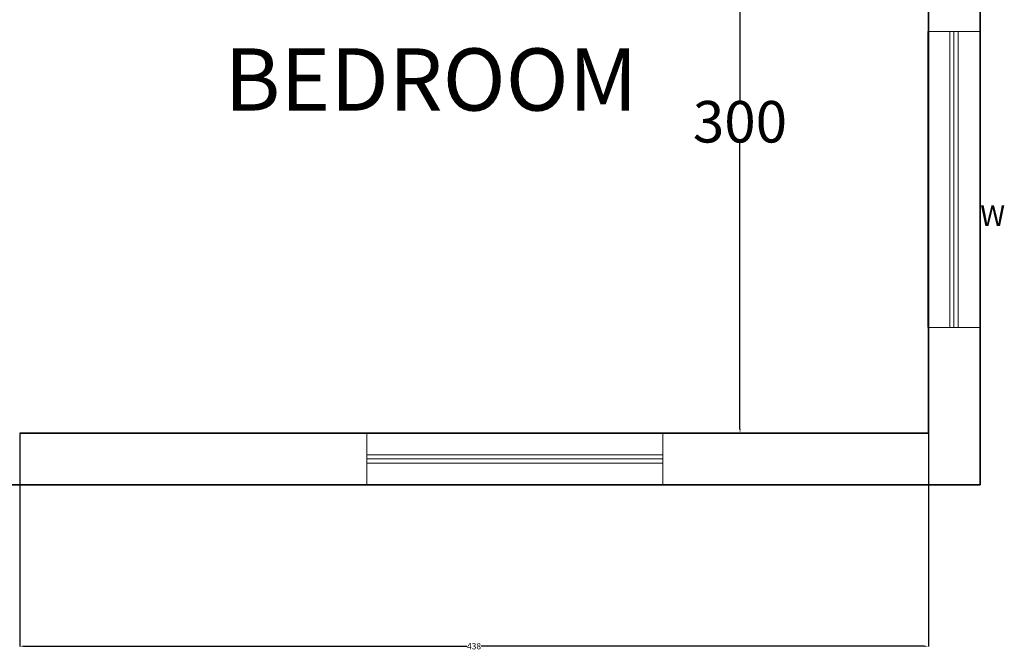
# Model space of a CAD drawing. Units: centimetres. Extents: x -121 to 3851, y -16 to 1180.
# Tile 14 of 16: x 3304 to 3779, y 16 to 320. Entities that reach past the tile are written whole.
import ezdxf

# ---------------------------------------------------------------- set-up
doc = ezdxf.new("R2010")
doc.units = ezdxf.units.CM
doc.header["$MEASUREMENT"] = 0
for name, color, linetype, lineweight in [('A-ANNO-DIMS', 2, 'Continuous', 18), ('A-ANNO-IDEN', 3, 'Continuous', 13), ('A-AREA-IDEN', 3, 'Continuous', 18), ('A-GLAZ', 4, 'Continuous', 18), ('A-WALL', 7, 'Continuous', 35)]:
    doc.layers.add(name, color=color, linetype=linetype, lineweight=lineweight)
doc.styles.get("Standard").update_dxf_attribs({"font": 'arial.ttf'})
doc.dimstyles.get("Standard").update_dxf_attribs({"dimtxt": 3, "dimasz": 2, "dimexe": 0.18, "dimexo": 0.0625, "dimgap": 0.09, "dimtad": 0, "dimtih": 1, "dimtoh": 1, "dimdec": 0, "dimzin": 0, "dimdsep": 46, "dimtxsty": 'Standard', "dimcen": 0.09, "dimadec": 0, "dimazin": 0, "dimtfac": 1, "dimtdec": 0, "dimtofl": 0, "dimtmove": 0, "dimatfit": 3, "dimfxl": 1, "dimtolj": 1, "dimtzin": 0, "dimarcsym": 0})

# ---------------------------------------------------------------- blocks, each defined once
blk = doc.blocks.new('*D17')
at = {"layer": 'A-ANNO-DIMS', "color": 0, "lineweight": -2, "transparency": 16777216}
for p, q in [((3651.46, 418.72), (3651.46, 281.03)), ((3651.53, 420.72), (3651.64, 420.72)), ((3651.46, 122.72), (3651.46, 260.41)), ((3651.53, 120.72), (3651.64, 120.72))]:
    blk.add_line(p, q, dxfattribs=at)
at = {"layer": 'A-ANNO-DIMS', "color": 0, "transparency": 16777216}
for points in [[(3651.13, 418.72), (3651.8, 418.72), (3651.46, 420.72)], [(3651.13, 122.72), (3651.8, 122.72), (3651.46, 120.72)]]:
    blk.add_solid(points, dxfattribs=at)
at = {"layer": 'Defpoints', "color": 0, "transparency": 16777216}
for p in [(3651.46, 420.72), (3651.46, 120.72), (3651.46, 120.72)]:
    blk.add_point(p, dxfattribs=at)
at = {"layer": 'A-ANNO-DIMS', "color": 0, "transparency": 16777216, "insert": (3651.46, 270.72), "char_height": 3, "attachment_point": 5}
blk.add_mtext('\\A1;{\\H6.66667x;300}', dxfattribs=at)
blk = doc.blocks.new('WIN-143CM')
for p, q in [((0, 14.5), (142.63, 14.5)), ((0, 12.5), (142.63, 12.5)), ((0, 10.5), (142.63, 10.5))]:
    blk.add_line(p, q)
blk.add_lwpolyline([(0, 25), (142.63, 25), (142.63, 0), (0, 0)], close=True)
blk = doc.blocks.new('*D64')
at = {"layer": 'A-ANNO-DIMS', "color": 0, "lineweight": -2, "transparency": 16777216}
for p, q in [((3304.26, 120.66), (3304.26, 17.79)), ((3742.26, 120.66), (3742.26, 17.79)), ((3306.26, 17.97), (3519.8, 17.97)), ((3740.26, 17.97), (3526.73, 17.97))]:
    blk.add_line(p, q, dxfattribs=at)
at = {"layer": 'A-ANNO-DIMS', "color": 0, "transparency": 16777216}
for points in [[(3306.26, 18.31), (3306.26, 17.64), (3304.26, 17.97)], [(3740.26, 18.31), (3740.26, 17.64), (3742.26, 17.97)]]:
    blk.add_solid(points, dxfattribs=at)
at = {"layer": 'Defpoints', "color": 0, "transparency": 16777216}
for p in [(3304.26, 120.72), (3742.26, 120.72), (3742.26, 17.97)]:
    blk.add_point(p, dxfattribs=at)
at = {"layer": 'A-ANNO-DIMS', "color": 0, "transparency": 16777216, "insert": (3523.26, 17.97), "char_height": 3, "attachment_point": 5}
blk.add_mtext('\\A1;438', dxfattribs=at)

msp = doc.modelspace()

# ---------------------------------------------------------------- linework, layer by layer
at = {"layer": 'A-WALL'}
for p, q in [((3767.2642, 911.7228), (3767.2642, 95.7228)), ((3742.2642, 420.7228), (3742.2642, 120.7228)), ((3742.2642, 120.7228), (3304.2642, 120.7228)), ((3767.2642, 95.7228), (2411.2642, 95.7228))]:
    msp.add_line(p, q, dxfattribs=at)

# ---------------------------------------------------------------- block references
at = {"layer": 'A-GLAZ', "rotation": 89.99999999999976}
msp.add_blockref('WIN-143CM', (3767.0732, 171.6176), dxfattribs=at)
at = {"layer": 'A-GLAZ'}
msp.add_blockref('WIN-143CM', (3471.6324, 95.7227), dxfattribs=at)

# ---------------------------------------------------------------- texts
at = {"layer": 'A-ANNO-IDEN', "insert": (3767.2642, 230.493), "char_height": 10, "attachment_point": 1}
msp.add_mtext_dynamic_manual_height_columns('W', width=55.718495, gutter_width=1, heights=[0], dxfattribs=at)
at = {"layer": 'A-AREA-IDEN', "insert": (3403.0289, 306.0859), "char_height": 30, "attachment_point": 1}
msp.add_mtext_dynamic_manual_height_columns('BEDROOM', width=248.976965, gutter_width=1, heights=[0], dxfattribs=at)

# ---------------------------------------------------------------- dimensions: what is measured, and where the dimension line sits
at = {"layer": 'A-ANNO-DIMS'}
dim = msp.add_linear_dim(base=(3651.464, 120.7228), p1=(3651.464, 420.7228), p2=(3651.464, 120.7228), angle=90, text='{\\H6.66667x;<>}', dimstyle='Standard', override={"dimclrd": 0, "dimclre": 0, "dimclrt": 0}, dxfattribs=at)
dim.commit()
dim.dimension.update_dxf_attribs({"geometry": '*D17', "text_midpoint": (3651.464, 270.7228)})
dim = msp.add_linear_dim(base=(3742.2642, 17.9728), p1=(3304.2642, 120.7228), p2=(3742.2642, 120.7228), dimstyle='Standard', override={"dimdec": 0, "dimlfac": 1, "dimrnd": 0, "dimzin": 0, "dimdsep": 46, "dimlunit": 2}, dxfattribs=at)
dim.commit()
dim.dimension.update_dxf_attribs({"geometry": '*D64', "text_midpoint": (3523.2642, 17.9728)})

doc.saveas('drawing.dxf')
